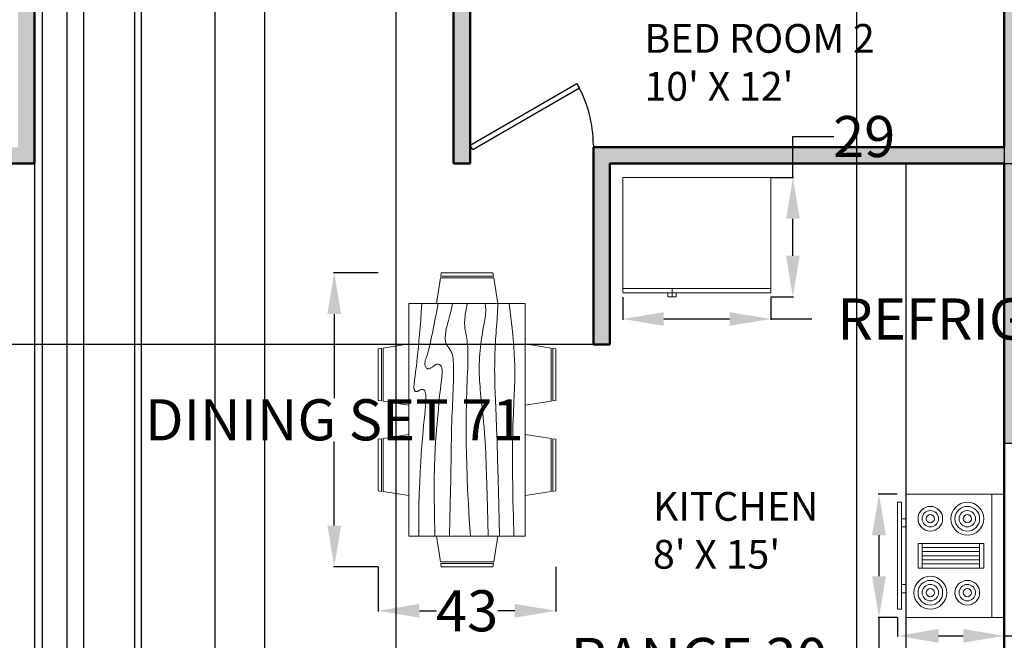
# Model space of a CAD drawing. Units: inches. Extents: x 133 to 758, y -29 to 543.
# Tile 5 of 7: x 386 to 626, y 235 to 386. Entities that reach past the tile are written whole.
import ezdxf

# ---------------------------------------------------------------- set-up
doc = ezdxf.new("R2010")
doc.units = ezdxf.units.IN
doc.header["$MEASUREMENT"] = 0
for name, color, linetype, lineweight in [('A-ANNO-DIMS', 2, 'Continuous', 18), ('A-AREA-IDEN', 7, 'Continuous', 25), ('A-EQPM', 8, 'Continuous', 20), ('A-FLOR-CASE', 32, 'Continuous', 25), ('A-FURN', 8, 'Continuous', 18), ('A-WALL', 7, 'Continuous', 50), ('DOOR', 40, 'Continuous', 25)]:
    doc.layers.add(name, color=color, linetype=linetype, lineweight=lineweight)
doc.layers.add('A-WALL-PATT', color=251, linetype='Continuous', lineweight=13, true_color=0x636466)
doc.styles.get("Standard").update_dxf_attribs({"font": 'arial.ttf'})
doc.dimstyles.get("Standard").update_dxf_attribs({"dimtxt": 10, "dimasz": 10, "dimexe": 0.18, "dimexo": 0.0625, "dimgap": 0.09, "dimtad": 0, "dimtih": 1, "dimtoh": 1, "dimdec": 0, "dimzin": 0, "dimdsep": 46, "dimlunit": 4, "dimtxsty": 'Standard', "dimcen": 0.09, "dimadec": 0, "dimazin": 0, "dimtfac": 1, "dimtdec": 0, "dimtofl": 0, "dimtmove": 0, "dimatfit": 3, "dimfxl": 1, "dimtolj": 1, "dimtzin": 0, "dimarcsym": 0})

# ---------------------------------------------------------------- blocks, each defined once
blk = doc.blocks.new('*U11')
for p, q in [((0, 0), (0, -6)), ((40, 0), (40, -6))]:
    blk.add_line(p, q)
blk.add_lwpolyline([(0, 0), (34.64, 20), (35.52, 18.48), (0.87, -1.52)], close=True)
blk.add_arc((0, 0), 40, 0, 30)
blk = doc.blocks.new('Range-Oven - 30 in top')
for p, q in [((0, -3), (30, -3)), ((12, -6), (18, -6)), ((13, -20), (13, -6)), ((14, -6), (14, -20)), ((15, -20), (15, -6)), ((16, -6), (16, -20)), ((17, -20), (17, -6)), ((18, -20), (12, -20)), ((6, -24), (6, -25)), ((8, -25), (8, -24)), ((22, -25), (22, -24)), ((24, -24), (24, -25))]:
    blk.add_line(p, q)
for points in [[(0, -24), (0, 0), (30, 0), (30, -24)], [(12, -21), (12, -5), (18, -5), (18, -21)], [(2, -26), (2, -25), (28, -25), (28, -26)]]:
    blk.add_lwpolyline(points, close=True)
for centre, radius in [((6, -9), 4), ((6, -9), 3), ((6, -9), 2), ((24, -9), 3), ((24, -9), 2), ((6, -9), 1), ((24, -9), 1), ((24, -18), 4), ((6, -18), 3), ((6, -18), 2), ((24, -18), 3), ((24, -18), 2), ((6, -18), 1), ((24, -18), 1)]:
    blk.add_circle(centre, radius)
blk = doc.blocks.new('Refrigerator-2 door - 36 in top')
for p, q in [((0, -26.999999), (36, -26.999999)), ((11, -27.999999), (11, -28.999999)), ((12, -26.999999), (12, -28.999999)), ((13, -28.999999), (13, -27.999999)), ((11, -28.999999), (13, -28.999999))]:
    blk.add_line(p, q)
blk.add_lwpolyline([(0, -27.999999), (0, 0), (36, 0), (36, -27.999999)], close=True)
blk = doc.blocks.new('Dining Set - 36 x 72 in.')
for p, q in [((-22, 27.5), (-22.1562, 26.50042)), ((-22, 27.5), (-6, 27.5)), ((-5.8437, 26.49966), (-6, 27.5)), ((6, 27.5), (5.8438, 26.50042)), ((6, 27.5), (22, 27.5)), ((22.1563, 26.49966), (22, 27.5)), ((-22.2343, 26.00059), (-23.4847, 17.99762)), ((-22.2304, 26), (-5.7608, 26)), ((-5.8416, 26.5), (-22.1534, 26.5)), ((-4.5152, 17.99762), (-5.7655, 25.99926)), ((5.7657, 26.00059), (4.5153, 17.99762)), ((5.7696, 26), (22.2392, 26)), ((22.1584, 26.5), (5.8466, 26.5)), ((23.4848, 17.99762), (22.2345, 25.99926)), ((36, 18), (-36, 18)), ((-36, 18), (-36, -18)), ((36, -18), (36, 18)), ((-44.0006, 8.23428), (-35.9976, 9.48474)), ((44.0006, 8.23428), (35.9976, 9.48474)), ((-45.5, 8), (-44.5004, 8.15617)), ((-45.5, 8), (-45.5, -8)), ((-44.5, -8.15843), (-44.5, 8.15338)), ((-44, 8.23041), (-44, -8.23915)), ((44, 8.23041), (44, -8.23915)), ((44.5, -8.15843), (44.5, 8.15338)), ((45.5, 8), (44.5005, 8.15617)), ((45.5, 8), (45.5, -8)), ((-44.4997, -8.15631), (-45.5, -8)), ((-35.9976, -9.48476), (-43.9993, -8.2345)), ((35.9976, -9.48476), (43.9993, -8.2345)), ((44.4997, -8.15631), (45.5, -8)), ((-36, -18), (36, -18)), ((-22.2343, -26.0006), (-23.4847, -17.99762)), ((-4.5152, -17.99762), (-5.7655, -25.99928)), ((5.7657, -26.0006), (4.5153, -17.99762)), ((23.4848, -17.99762), (22.2345, -25.99928)), ((-22.2304, -26), (-5.7608, -26)), ((-22, -27.5), (-22.1562, -26.50044)), ((-5.8416, -26.5), (-22.1534, -26.5)), ((-5.8437, -26.49967), (-6, -27.5)), ((5.7696, -26), (22.2392, -26)), ((6, -27.5), (5.8438, -26.50044)), ((22.1584, -26.5), (5.8466, -26.5)), ((22.1563, -26.49967), (22, -27.5)), ((-22, -27.5), (-6, -27.5)), ((6, -27.5), (22, -27.5))]:
    blk.add_line(p, q)
for points in [[(-36, 15), (-31.1772, 14.97754), (-26.8079, 14.91406), (-22.8538, 14.81543), (-19.276, 14.6875), (-16.0362, 14.53613), (-13.0957, 14.36718), (-10.4159, 14.18652), (-7.9583, 14), (-5.6904, 13.81315), (-3.6035, 13.63021), (-1.6954, 13.45508), (0.0365, 13.29166), (1.5945, 13.14388), (2.9811, 13.01562), (4.1988, 12.9108), (5.25, 12.83333), (6.1393, 12.78613), (6.8802, 12.76823), (7.4883, 12.77767), (7.9792, 12.8125), (8.3685, 12.87077), (8.6719, 12.95052), (8.9049, 13.0498), (9.0833, 13.16666), (9.2205, 13.29899), (9.3216, 13.44401), (9.3895, 13.59879), (9.4271, 13.76041), (9.4373, 13.92594), (9.4232, 14.09245), (9.3875, 14.257), (9.3333, 14.41666), (9.2638, 14.56917), (9.1836, 14.71484), (9.0975, 14.85465), (9.0104, 14.98958), (8.9272, 15.1206), (8.8529, 15.2487), (8.7922, 15.37483), (8.75, 15.5), (8.7305, 15.62467), (8.7344, 15.74739), (8.7617, 15.86621), (8.8125, 15.97916), (8.8867, 16.08431), (8.9844, 16.17968), (9.1055, 16.26334), (9.25, 16.33333), (9.4189, 16.38802), (9.6172, 16.42708), (9.8506, 16.45052), (10.125, 16.45833), (10.4463, 16.45052), (10.8203, 16.42708), (11.2529, 16.38802), (11.75, 16.33333), (12.3184, 16.26318), (12.9694, 16.17838), (13.7151, 16.07991), (14.5677, 15.96875), (15.5395, 15.84586), (16.6426, 15.71224), (17.8893, 15.56884), (19.2917, 15.41666), (20.859, 15.25667), (22.5879, 15.08984), (24.4721, 14.91715), (26.5052, 14.73958), (28.6809, 14.5581), (30.9929, 14.3737), (33.4347, 14.18733), (36, 14)], [(-36, 10), (-28.9766, 10.14274), (-23.1725, 10.20442), (-18.4241, 10.19775), (-14.5677, 10.13541), (-11.4399, 10.03011), (-8.877, 9.89453), (-6.7154, 9.74137), (-4.7917, 9.58333), (-2.9698, 9.43082), (-1.2246, 9.28515), (0.4415, 9.14534), (2.026, 9.01041), (3.5266, 8.87939), (4.9408, 8.7513), (6.266, 8.62516), (7.5, 8.5), (8.6411, 8.37549), (9.6914, 8.2539), (10.6538, 8.13818), (11.5312, 8.03125), (12.3267, 7.93603), (13.043, 7.85547), (13.6831, 7.79248), (14.25, 7.75), (14.7471, 7.7303), (15.1797, 7.73307), (15.5537, 7.75732), (15.875, 7.80208), (16.1494, 7.86637), (16.3828, 7.94922), (16.5811, 8.04964), (16.75, 8.16666), (16.8944, 8.29915), (17.0143, 8.44531), (17.1089, 8.60319), (17.1771, 8.77083), (17.218, 8.94629), (17.2305, 9.1276), (17.2137, 9.31282), (17.1667, 9.5), (17.0895, 9.6875), (16.987, 9.875), (16.8649, 10.0625), (16.7292, 10.25), (16.5856, 10.4375), (16.4401, 10.625), (16.2985, 10.8125), (16.1667, 11), (16.05, 11.18733), (15.9518, 11.3737), (15.8752, 11.5581), (15.8229, 11.73958), (15.798, 11.91715), (15.8034, 12.08984), (15.842, 12.25667), (15.9167, 12.41666), (16.0295, 12.56836), (16.1784, 12.70833), (16.3605, 12.83268), (16.5729, 12.9375), (16.8127, 13.01888), (17.0768, 13.07291), (17.3625, 13.0957), (17.6667, 13.08333), (17.9894, 13.03312), (18.3418, 12.94726), (18.7382, 12.82918), (19.1927, 12.68229), (19.7195, 12.51001), (20.3327, 12.31575), (21.0465, 12.10294), (21.875, 11.875), (22.8357, 11.63354), (23.959, 11.37304), (25.2786, 11.08618), (26.8282, 10.76562), (28.6414, 10.40405), (30.752, 9.99414), (33.1936, 9.52856), (36, 9)], [(-36, 5.5), (-30.7157, 5.3348), (-26.069, 5.20963), (-21.9946, 5.11767), (-18.4271, 5.05208), (-15.3009, 5.00602), (-12.5508, 4.97265), (-10.1112, 4.94515), (-7.9167, 4.91666), (-5.909, 4.88167), (-4.0586, 4.83984), (-2.3429, 4.79215), (-0.7396, 4.73958), (0.7739, 4.6831), (2.22, 4.6237), (3.6213, 4.56233), (5, 4.5), (6.373, 4.43782), (7.7344, 4.3776), (9.0723, 4.32129), (10.375, 4.27083), (11.6309, 4.22819), (12.8281, 4.19531), (13.9551, 4.17415), (15, 4.16666), (15.954, 4.17448), (16.819, 4.19791), (17.6001, 4.23698), (18.3021, 4.29166), (18.9299, 4.36198), (19.4883, 4.44791), (19.9823, 4.54948), (20.4167, 4.66666), (20.7969, 4.79899), (21.1302, 4.94401), (21.4245, 5.09879), (21.6875, 5.26041), (21.9271, 5.42594), (22.1511, 5.59245), (22.3672, 5.757), (22.5834, 5.91666), (22.8065, 6.06868), (23.0404, 6.21093), (23.2879, 6.34147), (23.5521, 6.45833), (23.8358, 6.55957), (24.142, 6.64323), (24.4735, 6.70735), (24.8334, 6.75), (25.2235, 6.76969), (25.642, 6.76692), (26.0858, 6.74267), (26.5521, 6.69791), (27.0379, 6.63362), (27.5404, 6.55078), (28.0565, 6.45036), (28.5834, 6.33333), (29.1242, 6.19987), (29.7071, 6.04687), (30.3661, 5.87044), (31.1354, 5.66666), (32.0493, 5.43164), (33.142, 5.16146), (34.4475, 4.85221), (36, 4.5)], [(-36, -1), (-30.7915, -0.6591), (-26.0195, -0.38216), (-21.6519, -0.16284), (-17.6563, 0.00521), (-14.0005, 0.12833), (-10.6523, 0.21289), (-7.5796, 0.26522), (-4.75, 0.29166), (-2.134, 0.29793), (0.2878, 0.28711), (2.5317, 0.26163), (4.6146, 0.22396), (6.5529, 0.17651), (8.3633, 0.12174), (10.0623, 0.06209), (11.6667, 0), (13.1899, -0.06201), (14.6341, -0.1211), (15.9982, -0.17432), (17.2813, -0.21875), (18.4823, -0.25147), (19.6003, -0.26953), (20.6343, -0.27002), (21.5834, -0.25), (22.4481, -0.20768), (23.2357, -0.14584), (23.9549, -0.06836), (24.6146, 0.02083), (25.2235, 0.11784), (25.7904, 0.21875), (26.3241, 0.31966), (26.8334, 0.41666), (27.3265, 0.50618), (27.8099, 0.58593), (28.2894, 0.65397), (28.7709, 0.70833), (29.2601, 0.74707), (29.763, 0.76823), (30.2855, 0.76985), (30.8334, 0.75), (31.4088, 0.70784), (31.9994, 0.64713), (32.589, 0.57275), (33.1615, 0.48958), (33.7008, 0.4025), (34.1908, 0.3164), (34.6153, 0.23616), (34.9584, 0.16666), (35.2099, 0.11165), (35.3848, 0.07031), (35.504, 0.04069), (35.5886, 0.02083), (35.6594, 0.00879), (35.7377, 0.0026), (35.8442, 0.00032), (36, 0)], [(-36, -6.5), (-27.1843, -6.31267), (-20.084, -6.1263), (-14.469, -5.9419), (-10.1094, -5.76042), (-6.7752, -5.58285), (-4.2363, -5.41016), (-2.2629, -5.24333), (-0.625, -5.08334), (0.8708, -4.93099), (2.2715, -4.78646), (3.5872, -4.64974), (4.8281, -4.52084), (6.0046, -4.39974), (7.127, -4.28646), (8.2053, -4.18099), (9.25, -4.08334), (10.2705, -3.99382), (11.2734, -3.91407), (12.2647, -3.84603), (13.25, -3.79167), (14.2354, -3.75293), (15.2266, -3.73177), (16.2295, -3.73015), (17.25, -3.75), (18.2912, -3.79248), (19.3451, -3.85547), (20.4009, -3.93604), (21.4479, -4.03125), (22.4754, -4.13819), (23.4727, -4.25391), (24.4289, -4.37549), (25.3334, -4.5), (26.1785, -4.62492), (26.9694, -4.74935), (27.7145, -4.87281), (28.4219, -4.99479), (29.1, -5.11483), (29.7572, -5.23242), (30.4016, -5.34709), (31.0417, -5.45834), (31.6837, -5.56437), (32.3262, -5.65821), (32.9658, -5.73153), (33.599, -5.77604), (34.2224, -5.78345), (34.8327, -5.74545), (35.4264, -5.65373), (36, -5.5)], [(-36, -10), (-26.4022, -9.81299), (-18.4675, -9.62891), (-11.9839, -9.45069), (-6.7396, -9.28125), (-2.5226, -9.12354), (0.8789, -8.98047), (3.6769, -8.85498), (6.0833, -8.75), (8.2767, -8.66765), (10.3021, -8.60677), (12.1712, -8.56543), (13.8958, -8.54167), (15.4876, -8.53353), (16.9583, -8.53907), (18.3197, -8.55632), (19.5834, -8.58334), (20.7616, -8.61841), (21.8685, -8.66081), (22.9188, -8.71004), (23.9271, -8.76563), (24.9081, -8.82707), (25.8763, -8.89388), (26.8465, -8.96558), (27.8334, -9.04167), (28.8474, -9.12118), (29.8828, -9.20117), (30.93, -9.27824), (31.9792, -9.34896), (33.0205, -9.40991), (34.0443, -9.45768), (35.0407, -9.48885), (36, -9.5)], [(-36, -14.5), (-30.0881, -14.33513), (-25.0332, -14.21224), (-20.7312, -14.12647), (-17.0781, -14.07292), (-13.97, -14.04671), (-11.3027, -14.04297), (-8.9724, -14.05681), (-6.875, -14.08334), (-4.9224, -14.11833), (-3.0905, -14.16016), (-1.3709, -14.20785), (0.2448, -14.26042), (1.7647, -14.3169), (3.1973, -14.3763), (4.5507, -14.43767), (5.8333, -14.5), (7.0554, -14.5621), (8.235, -14.62175), (9.3922, -14.67652), (10.5469, -14.72396), (11.7192, -14.76164), (12.929, -14.78711), (14.1965, -14.79794), (15.5417, -14.79167), (16.9933, -14.76424), (18.6152, -14.70508), (20.4804, -14.60197), (22.6615, -14.44271), (25.2312, -14.21509), (28.2624, -13.9069), (31.8277, -13.50594), (36, -13)]]:
    blk.add_lwpolyline(points)
blk = doc.blocks.new('*D44')
at = {"layer": 'A-ANNO-DIMS', "color": 0, "lineweight": -2, "transparency": 16777216}
for p, q in [((538.86, 405.84), (538.86, 393.72)), ((618.86, 405.84), (618.86, 393.72)), ((548.86, 393.9), (608.86, 393.9)), ((618.86, 393.9), (628.86, 393.9))]:
    blk.add_line(p, q, dxfattribs=at)
at = {"layer": 'A-ANNO-DIMS', "color": 0, "transparency": 16777216}
for points in [[(548.86, 395.56), (548.86, 392.23), (538.86, 393.9)], [(608.86, 395.56), (608.86, 392.23), (618.86, 393.9)]]:
    blk.add_solid(points, dxfattribs=at)
at = {"layer": 'Defpoints', "color": 0, "transparency": 16777216}
for p in [(538.86, 405.9), (618.86, 405.9), (618.86, 393.9)]:
    blk.add_point(p, dxfattribs=at)
at = {"layer": 'A-ANNO-DIMS', "color": 0, "transparency": 16777216, "insert": (696.36, 393.9), "char_height": 10, "attachment_point": 5}
blk.add_mtext('\\A1;QUEEN BED 80 TYP.', dxfattribs=at)
blk = doc.blocks.new('*D62')
at = {"layer": 'A-ANNO-DIMS', "color": 0, "lineweight": -2, "transparency": 16777216}
for p, q in [((599.69, 270.92), (595.07, 270.92)), ((595.25, 260.92), (595.25, 250.92)), ((599.69, 240.92), (595.07, 240.92)), ((595.25, 240.92), (595.25, 230.92)), ((595.25, 230.92), (585.25, 230.92))]:
    blk.add_line(p, q, dxfattribs=at)
at = {"layer": 'A-ANNO-DIMS', "color": 0, "transparency": 16777216}
for points in [[(593.58, 260.92), (596.92, 260.92), (595.25, 270.92)], [(593.58, 250.92), (596.92, 250.92), (595.25, 240.92)]]:
    blk.add_solid(points, dxfattribs=at)
at = {"layer": 'Defpoints', "color": 0, "transparency": 16777216}
for p in [(599.75, 270.92), (595.25, 240.92), (599.75, 240.92)]:
    blk.add_point(p, dxfattribs=at)
at = {"layer": 'A-ANNO-DIMS', "color": 0, "transparency": 16777216, "insert": (551.49, 230.92), "char_height": 10, "attachment_point": 5}
blk.add_mtext('\\A1;RANGE 30', dxfattribs=at)
blk = doc.blocks.new('*D63')
at = {"layer": 'A-ANNO-DIMS', "color": 0, "lineweight": -2, "transparency": 16777216}
for p, q in [((599.75, 240.86), (599.75, 236.24)), ((625.75, 240.86), (625.75, 236.24)), ((609.75, 236.42), (615.75, 236.42)), ((625.75, 236.42), (635.75, 236.42))]:
    blk.add_line(p, q, dxfattribs=at)
at = {"layer": 'A-ANNO-DIMS', "color": 0, "transparency": 16777216}
for points in [[(609.75, 238.09), (609.75, 234.75), (599.75, 236.42)], [(615.75, 238.09), (615.75, 234.75), (625.75, 236.42)]]:
    blk.add_solid(points, dxfattribs=at)
at = {"layer": 'Defpoints', "color": 0, "transparency": 16777216}
for p in [(599.75, 240.92), (625.75, 240.92), (625.75, 236.42)]:
    blk.add_point(p, dxfattribs=at)
at = {"layer": 'A-ANNO-DIMS', "color": 0, "transparency": 16777216, "insert": (643.08, 236.42), "char_height": 10, "attachment_point": 5}
blk.add_mtext('\\A1;26', dxfattribs=at)
blk = doc.blocks.new('*D66')
at = {"layer": 'A-ANNO-DIMS', "color": 0, "lineweight": -2, "transparency": 16777216}
for p, q in [((532.9, 318.87), (532.9, 313.35)), ((568.9, 318.87), (568.9, 313.35)), ((542.9, 313.53), (558.9, 313.53)), ((568.9, 313.53), (578.9, 313.53))]:
    blk.add_line(p, q, dxfattribs=at)
at = {"layer": 'A-ANNO-DIMS', "color": 0, "transparency": 16777216}
for points in [[(542.9, 315.2), (542.9, 311.86), (532.9, 313.53)], [(558.9, 315.2), (558.9, 311.86), (568.9, 313.53)]]:
    blk.add_solid(points, dxfattribs=at)
at = {"layer": 'Defpoints', "color": 0, "transparency": 16777216}
for p in [(532.9, 318.93), (568.9, 318.93), (568.9, 313.53)]:
    blk.add_point(p, dxfattribs=at)
at = {"layer": 'A-ANNO-DIMS', "color": 0, "transparency": 16777216, "insert": (643.33, 313.53), "char_height": 10, "attachment_point": 5}
blk.add_mtext('\\A1;REFRIGERATOR 36', dxfattribs=at)
blk = doc.blocks.new('*D67')
at = {"layer": 'A-ANNO-DIMS', "color": 0, "lineweight": -2, "transparency": 16777216}
for p, q in [((574.3, 347.93), (574.3, 357.93)), ((574.3, 357.93), (584.3, 357.93)), ((568.97, 347.93), (574.48, 347.93)), ((574.3, 328.93), (574.3, 337.93)), ((568.97, 318.93), (574.48, 318.93))]:
    blk.add_line(p, q, dxfattribs=at)
at = {"layer": 'A-ANNO-DIMS', "color": 0, "transparency": 16777216}
for points in [[(572.64, 337.93), (575.97, 337.93), (574.3, 347.93)], [(572.64, 328.93), (575.97, 328.93), (574.3, 318.93)]]:
    blk.add_solid(points, dxfattribs=at)
at = {"layer": 'Defpoints', "color": 0, "transparency": 16777216}
for p in [(568.9, 347.93), (574.3, 347.93), (568.9, 318.93)]:
    blk.add_point(p, dxfattribs=at)
at = {"layer": 'A-ANNO-DIMS', "color": 0, "transparency": 16777216, "insert": (591.65, 357.93), "char_height": 10, "attachment_point": 5}
blk.add_mtext('\\A1;29', dxfattribs=at)
blk = doc.blocks.new('*D68')
at = {"layer": 'A-ANNO-DIMS', "color": 0, "lineweight": -2, "transparency": 16777216}
for p, q in [((473.36, 324.74), (462.52, 324.74)), ((462.7, 314.74), (462.7, 294.25)), ((462.7, 263.25), (462.7, 283.73)), ((473.36, 253.25), (462.52, 253.25))]:
    blk.add_line(p, q, dxfattribs=at)
at = {"layer": 'A-ANNO-DIMS', "color": 0, "transparency": 16777216}
for points in [[(461.04, 314.74), (464.37, 314.74), (462.7, 324.74)], [(461.04, 263.25), (464.37, 263.25), (462.7, 253.25)]]:
    blk.add_solid(points, dxfattribs=at)
at = {"layer": 'Defpoints', "color": 0, "transparency": 16777216}
for p in [(462.7, 324.74), (473.43, 324.74), (473.43, 253.25)]:
    blk.add_point(p, dxfattribs=at)
at = {"layer": 'A-ANNO-DIMS', "color": 0, "transparency": 16777216, "insert": (462.7, 288.99), "char_height": 10, "attachment_point": 5}
blk.add_mtext('\\A1;DINING SET 71', dxfattribs=at)
blk = doc.blocks.new('*D69')
at = {"layer": 'A-ANNO-DIMS', "color": 0, "lineweight": -2, "transparency": 16777216}
for p, q in [((473.43, 253.18), (473.43, 242.34)), ((516.64, 253.18), (516.64, 242.34)), ((483.43, 242.52), (487.58, 242.52)), ((506.64, 242.52), (502.49, 242.52))]:
    blk.add_line(p, q, dxfattribs=at)
at = {"layer": 'A-ANNO-DIMS', "color": 0, "transparency": 16777216}
for points in [[(483.43, 244.19), (483.43, 240.85), (473.43, 242.52)], [(506.64, 244.19), (506.64, 240.85), (516.64, 242.52)]]:
    blk.add_solid(points, dxfattribs=at)
at = {"layer": 'Defpoints', "color": 0, "transparency": 16777216}
for p in [(473.43, 253.25), (516.64, 253.25), (473.43, 242.52)]:
    blk.add_point(p, dxfattribs=at)
at = {"layer": 'A-ANNO-DIMS', "color": 0, "transparency": 16777216, "insert": (495.03, 242.52), "char_height": 10, "attachment_point": 5}
blk.add_mtext('\\A1;43', dxfattribs=at)
blk = doc.blocks.new('*D75')
at = {"layer": 'A-ANNO-DIMS', "color": 0, "lineweight": -2, "transparency": 16777216}
for p, q in [((525.69, 307.34), (231.17, 307.34)), ((231.35, 297.34), (231.35, 264.53)), ((231.35, 221.34), (231.35, 254.14)), ((525.69, 211.34), (231.17, 211.34))]:
    blk.add_line(p, q, dxfattribs=at)
at = {"layer": 'A-ANNO-DIMS', "color": 0, "transparency": 16777216}
for points in [[(229.68, 297.34), (233.02, 297.34), (231.35, 307.34)], [(229.68, 221.34), (233.02, 221.34), (231.35, 211.34)]]:
    blk.add_solid(points, dxfattribs=at)
at = {"layer": 'Defpoints', "color": 0, "transparency": 16777216}
for p in [(231.35, 307.34), (525.75, 307.34), (525.75, 211.34)]:
    blk.add_point(p, dxfattribs=at)
at = {"layer": 'A-ANNO-DIMS', "color": 0, "transparency": 16777216, "insert": (231.35, 259.34), "char_height": 10, "attachment_point": 5}
blk.add_mtext('\\A1;96', dxfattribs=at)
blk = doc.blocks.new('*D78')
at = {"layer": 'A-ANNO-DIMS', "color": 0, "lineweight": -2, "transparency": 16777216}
for p, q in [((361.75, 167.4), (361.75, 533.92)), ((371.75, 533.74), (381.75, 533.74)), ((391.75, 167.4), (391.75, 533.92)), ((391.75, 533.74), (401.75, 533.74))]:
    blk.add_line(p, q, dxfattribs=at)
at = {"layer": 'A-ANNO-DIMS', "color": 0, "transparency": 16777216}
for points in [[(371.75, 535.4), (371.75, 532.07), (361.75, 533.74)], [(381.75, 535.4), (381.75, 532.07), (391.75, 533.74)]]:
    blk.add_solid(points, dxfattribs=at)
at = {"layer": 'Defpoints', "color": 0, "transparency": 16777216}
for p in [(391.75, 533.74), (361.75, 167.34), (391.75, 167.34)]:
    blk.add_point(p, dxfattribs=at)
at = {"layer": 'A-ANNO-DIMS', "color": 0, "transparency": 16777216, "insert": (408.98, 533.74), "char_height": 10, "attachment_point": 5}
blk.add_mtext('\\A1;30', dxfattribs=at)
blk = doc.blocks.new('*D81')
at = {"layer": 'A-ANNO-DIMS', "color": 0, "lineweight": -2, "transparency": 16777216}
for p, q in [((589.75, 499.27), (589.75, -22.24)), ((625.75, 499.27), (625.75, -22.24)), ((599.75, -22.06), (600.5, -22.06)), ((615.75, -22.06), (615, -22.06))]:
    blk.add_line(p, q, dxfattribs=at)
at = {"layer": 'A-ANNO-DIMS', "color": 0, "transparency": 16777216}
for points in [[(599.75, -20.4), (599.75, -23.73), (589.75, -22.06)], [(615.75, -20.4), (615.75, -23.73), (625.75, -22.06)]]:
    blk.add_solid(points, dxfattribs=at)
at = {"layer": 'Defpoints', "color": 0, "transparency": 16777216}
for p in [(589.75, 499.34), (625.75, 499.34), (625.75, -22.06)]:
    blk.add_point(p, dxfattribs=at)
at = {"layer": 'A-ANNO-DIMS', "color": 0, "transparency": 16777216, "insert": (607.75, -22.06), "char_height": 10, "attachment_point": 5}
blk.add_mtext('\\A1;36', dxfattribs=at)
blk = doc.blocks.new('*D82')
at = {"layer": 'A-ANNO-DIMS', "color": 0, "lineweight": -2, "transparency": 16777216}
for p, q in [((625.81, 351.34), (660.33, 351.34)), ((660.15, 341.34), (660.15, 322.53)), ((660.15, 293.34), (660.15, 312.14)), ((625.81, 283.34), (660.33, 283.34))]:
    blk.add_line(p, q, dxfattribs=at)
at = {"layer": 'A-ANNO-DIMS', "color": 0, "transparency": 16777216}
for points in [[(658.48, 341.34), (661.82, 341.34), (660.15, 351.34)], [(658.48, 293.34), (661.82, 293.34), (660.15, 283.34)]]:
    blk.add_solid(points, dxfattribs=at)
at = {"layer": 'Defpoints', "color": 0, "transparency": 16777216}
for p in [(625.75, 351.34), (625.75, 283.34), (660.15, 283.34)]:
    blk.add_point(p, dxfattribs=at)
at = {"layer": 'A-ANNO-DIMS', "color": 0, "transparency": 16777216, "insert": (660.15, 317.34), "char_height": 10, "attachment_point": 5}
blk.add_mtext('\\A1;68', dxfattribs=at)
blk = doc.blocks.new('*D85')
at = {"layer": 'A-ANNO-DIMS', "color": 0, "lineweight": -2, "transparency": 16777216}
for p, q in [((389.75, 399.27), (389.75, -22.24)), ((415.75, 399.27), (415.75, -22.24)), ((389.75, -22.06), (379.75, -22.06)), ((405.75, -22.06), (399.75, -22.06))]:
    blk.add_line(p, q, dxfattribs=at)
at = {"layer": 'A-ANNO-DIMS', "color": 0, "transparency": 16777216}
for points in [[(399.75, -20.4), (399.75, -23.73), (389.75, -22.06)], [(405.75, -20.4), (405.75, -23.73), (415.75, -22.06)]]:
    blk.add_solid(points, dxfattribs=at)
at = {"layer": 'Defpoints', "color": 0, "transparency": 16777216}
for p in [(389.75, 399.34), (415.75, 399.34), (389.75, -22.06)]:
    blk.add_point(p, dxfattribs=at)
at = {"layer": 'A-ANNO-DIMS', "color": 0, "transparency": 16777216, "insert": (372.42, -22.06), "char_height": 10, "attachment_point": 5}
blk.add_mtext('\\A1;26', dxfattribs=at)
blk = doc.blocks.new('*D89')
at = {"layer": 'A-ANNO-DIMS', "color": 0, "lineweight": -2, "transparency": 16777216}
for p, q in [((387.75, 533.74), (377.75, 533.74)), ((397.75, 163.4), (397.75, 533.92)), ((401.75, 163.4), (401.75, 533.92)), ((411.75, 533.74), (421.75, 533.74))]:
    blk.add_line(p, q, dxfattribs=at)
at = {"layer": 'A-ANNO-DIMS', "color": 0, "transparency": 16777216}
for points in [[(387.75, 535.4), (387.75, 532.07), (397.75, 533.74)], [(411.75, 535.4), (411.75, 532.07), (401.75, 533.74)]]:
    blk.add_solid(points, dxfattribs=at)
at = {"layer": 'Defpoints', "color": 0, "transparency": 16777216}
for p in [(401.75, 533.74), (397.75, 163.34), (401.75, 163.34)]:
    blk.add_point(p, dxfattribs=at)
at = {"layer": 'A-ANNO-DIMS', "color": 0, "transparency": 16777216, "insert": (425.3, 533.74), "char_height": 10, "attachment_point": 5}
blk.add_mtext('\\A1;4', dxfattribs=at)
blk = doc.blocks.new('*D90')
at = {"layer": 'A-ANNO-DIMS', "color": 0, "lineweight": -2, "transparency": 16777216}
for p, q in [((433.75, 167.4), (433.75, 533.92)), ((443.75, 533.74), (448.32, 533.74)), ((467.75, 533.74), (463.18, 533.74)), ((477.75, 163.4), (477.75, 533.92))]:
    blk.add_line(p, q, dxfattribs=at)
at = {"layer": 'A-ANNO-DIMS', "color": 0, "transparency": 16777216}
for points in [[(443.75, 535.4), (443.75, 532.07), (433.75, 533.74)], [(467.75, 535.4), (467.75, 532.07), (477.75, 533.74)]]:
    blk.add_solid(points, dxfattribs=at)
at = {"layer": 'Defpoints', "color": 0, "transparency": 16777216}
for p in [(477.75, 533.74), (433.75, 167.34), (477.75, 163.34)]:
    blk.add_point(p, dxfattribs=at)
at = {"layer": 'A-ANNO-DIMS', "color": 0, "transparency": 16777216, "insert": (455.75, 533.74), "char_height": 10, "attachment_point": 5}
blk.add_mtext('\\A1;44', dxfattribs=at)
blk = doc.blocks.new('*D91')
at = {"layer": 'A-ANNO-DIMS', "color": 0, "lineweight": -2, "transparency": 16777216}
for p, q in [((415.75, 399.27), (415.75, -22.24)), ((445.75, 399.27), (445.75, -22.24)), ((425.75, -22.06), (435.75, -22.06)), ((445.75, -22.06), (455.75, -22.06))]:
    blk.add_line(p, q, dxfattribs=at)
at = {"layer": 'A-ANNO-DIMS', "color": 0, "transparency": 16777216}
for points in [[(425.75, -20.4), (425.75, -23.73), (415.75, -22.06)], [(435.75, -20.4), (435.75, -23.73), (445.75, -22.06)]]:
    blk.add_solid(points, dxfattribs=at)
at = {"layer": 'Defpoints', "color": 0, "transparency": 16777216}
for p in [(415.75, 399.34), (445.75, 399.34), (445.75, -22.06)]:
    blk.add_point(p, dxfattribs=at)
at = {"layer": 'A-ANNO-DIMS', "color": 0, "transparency": 16777216, "insert": (462.98, -22.06), "char_height": 10, "attachment_point": 5}
blk.add_mtext('\\A1;30', dxfattribs=at)
blk = doc.blocks.new('*D99')
at = {"layer": 'A-ANNO-DIMS', "color": 0, "lineweight": -2, "transparency": 16777216}
for p, q in [((391.75, 533.74), (381.75, 533.74)), ((401.75, 19.4), (401.75, 533.92)), ((414.17, 21.95), (414.17, 533.92)), ((424.17, 533.74), (434.17, 533.74))]:
    blk.add_line(p, q, dxfattribs=at)
at = {"layer": 'A-ANNO-DIMS', "color": 0, "transparency": 16777216}
for points in [[(391.75, 535.4), (391.75, 532.07), (401.75, 533.74)], [(424.17, 535.4), (424.17, 532.07), (414.17, 533.74)]]:
    blk.add_solid(points, dxfattribs=at)
at = {"layer": 'Defpoints', "color": 0, "transparency": 16777216}
for p in [(401.75, 533.74), (414.17, 21.89), (401.75, 19.34)]:
    blk.add_point(p, dxfattribs=at)
at = {"layer": 'A-ANNO-DIMS', "color": 0, "transparency": 16777216, "insert": (361.37, 533.74), "char_height": 10, "attachment_point": 5}
blk.add_mtext('\\A1;12.417', dxfattribs=at)

msp = doc.modelspace()

# ---------------------------------------------------------------- hatches: boundary and pattern name
at = {"layer": 'A-WALL-PATT'}
h = msp.add_hatch(color=256, dxfattribs=at)
h.dxf.hatch_style = 1
h.paths.add_polyline_path([(433.7501, 508.336), (349.7501, 508.336), (349.7501, 499.336), (385.7501, 499.336), (385.7501, 403.336), (385.7501, 355.336), (379.7501, 355.336), (379.7501, 351.336), (389.7501, 351.336), (389.7501, 399.336), (415.7501, 399.336), (415.7501, 403.336), (389.7501, 403.336), (389.7501, 499.336), (433.7501, 499.336)])
h.paths.add_polyline_path([(541.7501, 508.336), (457.7501, 508.336), (457.7501, 499.336), (491.7501, 499.336), (491.7501, 403.336), (445.7501, 403.336), (445.7501, 399.336), (491.7501, 399.336), (491.7501, 351.336), (495.7501, 351.336), (495.7501, 399.336), (495.7501, 499.336), (513.7501, 499.336), (541.7501, 499.336)])
h.paths.add_polyline_path([(634.7501, 508.336), (589.7501, 508.336), (589.7501, 499.336), (625.7501, 499.336), (625.7501, 355.336), (525.7501, 355.336), (525.7501, 351.336), (525.7501, 307.336), (529.7501, 307.336), (529.7501, 351.336), (625.7501, 351.336), (625.7501, 283.336), (634.7501, 283.336)])
h.paths.add_polyline_path([(301.7501, 508.336), (256.7501, 508.336), (256.7501, 283.336), (265.7501, 283.336), (265.7501, 351.336), (349.7501, 351.336), (349.7501, 355.336), (265.7501, 355.336), (265.7501, 499.336), (301.7501, 499.336)])
h.paths.add_polyline_path([(361.7501, 167.336), (265.7501, 167.336), (265.7501, 235.336), (256.7501, 235.336), (256.7501, 10.336), (309.4362, 10.336), (309.4362, 19.336), (265.7501, 19.336), (265.7501, 163.336), (283.7501, 163.336), (361.7501, 163.336)])

# ---------------------------------------------------------------- linework, layer by layer
at = {"layer": 'A-FLOR-CASE'}
msp.add_line((601.7501, 351.336), (601.7501, 191.336), dxfattribs=at)
at = {"layer": 'A-WALL'}
for p, q in [((625.7501, 499.336), (625.7501, 355.336)), ((389.7501, 351.336), (389.7501, 399.336)), ((491.7501, 399.336), (491.7501, 351.336)), ((495.7501, 399.336), (495.7501, 351.336)), ((525.7501, 355.336), (625.7501, 355.336)), ((525.7501, 351.336), (525.7501, 355.336)), ((379.7501, 351.336), (389.7501, 351.336)), ((495.7501, 351.336), (491.7501, 351.336)), ((525.7501, 351.336), (525.7501, 307.336)), ((529.7501, 351.336), (529.7501, 307.336)), ((529.7501, 351.336), (625.7501, 351.336)), ((625.7501, 351.336), (625.7501, 167.336)), ((529.7501, 307.336), (525.7501, 307.336))]:
    msp.add_line(p, q, dxfattribs=at)

# ---------------------------------------------------------------- block references
at = {"layer": 'A-EQPM'}
msp.add_blockref('Refrigerator-2 door - 36 in top', (532.9033, 347.9301), dxfattribs=at)
at = {"layer": 'A-EQPM', "rotation": 270}
msp.add_blockref('Range-Oven - 30 in top', (625.7501, 270.9203), dxfattribs=at)
at = {"layer": 'A-FURN', "xscale": 0.7856607656645157, "yscale": 0.7856607656645157, "zscale": 0.7856607656645157, "rotation": 90}
msp.add_blockref('Dining Set - 36 x 72 in.', (495.0322, 288.9927), dxfattribs=at)
at = {"layer": 'DOOR', "xscale": 0.75, "yscale": 0.75, "zscale": 0.75}
msp.add_blockref('*U11', (495.7501, 355.836), dxfattribs=at)

# ---------------------------------------------------------------- texts
at = {"layer": 'A-AREA-IDEN', "char_height": 7, "attachment_point": 1}
for s, width, insert in [("BED ROOM 2 \\P10' X 12'", 109.09065, (538.1884, 385.3115)), ("KITCHEN\\P8' X 15'", 62.727145, (540.2554, 271.4286))]:
    msp.add_mtext_dynamic_manual_height_columns(s, width=width, gutter_width=1, heights=[0], dxfattribs=dict(at, insert=insert))

# ---------------------------------------------------------------- dimensions: what is measured, and where the dimension line sits
at = {"layer": 'A-ANNO-DIMS'}
for base, p1, p2, override, picture, middle in [((401.75012, 533.73604), (414.16755, 21.88596), (401.75012, 19.33604), {"dimdec": 3, "dimlfac": 1, "dimrnd": 0, "dimzin": 0, "dimdsep": 46, "dimlunit": 2}, '*D99', (361.37362, 533.73604)), ((391.7501, 533.736), (361.7501, 167.336), (391.7501, 167.336), {"dimdec": 0, "dimlfac": 1, "dimrnd": 0, "dimzin": 0, "dimdsep": 46, "dimlunit": 2}, '*D78', (408.982, 533.736)), ((401.7501, 533.736), (397.7501, 163.336), (401.7501, 163.336), {"dimdec": 0, "dimlfac": 1, "dimrnd": 0, "dimzin": 0, "dimdsep": 46, "dimlunit": 2}, '*D89', (425.2985, 533.736)), ((477.7501, 533.736), (433.7501, 167.336), (477.7501, 163.336), {"dimdec": 0, "dimlfac": 1, "dimrnd": 0, "dimzin": 0, "dimdsep": 46, "dimlunit": 2}, '*D90', (455.7501, 533.736)), ((625.7501, -22.064), (589.7501, 499.336), (625.7501, 499.336), {"dimdec": 0, "dimlfac": 1, "dimrnd": 0, "dimzin": 0, "dimdsep": 46, "dimlunit": 2}, '*D81', (607.7501, -22.064)), ((389.7501, -22.064), (415.7501, 399.336), (389.7501, 399.336), {"dimdec": 0, "dimlfac": 1, "dimrnd": 0, "dimzin": 0, "dimdsep": 46, "dimlunit": 2}, '*D85', (372.4159, -22.064)), ((445.7501, -22.064), (415.7501, 399.336), (445.7501, 399.336), {"dimdec": 0, "dimlfac": 1, "dimrnd": 0, "dimzin": 0, "dimdsep": 46, "dimlunit": 2}, '*D91', (462.982, -22.064)), ((625.7501, 236.4203), (599.7501, 240.9203), (625.7501, 240.9203), {"dimdec": 0, "dimlfac": 1, "dimrnd": 0, "dimzin": 0, "dimdsep": 46, "dimlunit": 2}, '*D63', (643.0843, 236.4203))]:
    dim = msp.add_linear_dim(base=base, p1=p1, p2=p2, dimstyle='Standard', override=override, dxfattribs=at)
    dim.commit()
    dim.dimension.update_dxf_attribs({"geometry": picture, "text_midpoint": middle})
for base, p1, p2, text, picture, middle in [((618.8575, 393.8976), (538.8574, 405.8976), (618.8575, 405.8976), 'QUEEN BED <> TYP.', '*D44', (696.3588, 393.8976)), ((568.9033, 313.5301), (532.9033, 318.9301), (568.9033, 318.9301), 'REFRIGERATOR <>', '*D66', (643.3282, 313.5301))]:
    dim = msp.add_linear_dim(base=base, p1=p1, p2=p2, text=text, dimstyle='Standard', override={"dimdec": 0, "dimlfac": 1, "dimrnd": 0, "dimzin": 0, "dimdsep": 46, "dimlunit": 2}, dxfattribs=at)
    dim.commit()
    dim.dimension.update_dxf_attribs({"geometry": picture, "text_midpoint": middle})
for base, p1, p2, angle, picture, middle in [((574.3033, 347.9301), (568.9033, 318.9301), (568.9033, 347.9301), 90, '*D67', (591.6511, 357.9301)), ((660.1501, 283.336), (625.7501, 351.336), (625.7501, 283.336), 90, '*D82', (660.1501, 317.336)), ((231.3501, 307.336), (525.7501, 211.336), (525.7501, 307.336), 90, '*D75', (231.3501, 259.336)), ((473.4265, 242.5208), (516.6379, 253.2451), (473.4265, 253.2451), 180, '*D69', (495.0322, 242.5208))]:
    dim = msp.add_linear_dim(base=base, p1=p1, p2=p2, angle=angle, dimstyle='Standard', override={"dimdec": 0, "dimlfac": 1, "dimrnd": 0, "dimzin": 0, "dimdsep": 46, "dimlunit": 2}, dxfattribs=at)
    dim.commit()
    dim.dimension.update_dxf_attribs({"geometry": picture, "text_midpoint": middle})
for base, p1, p2, angle, text, picture, middle in [((462.7023, 324.7402), (473.4265, 253.2451), (473.4265, 324.7402), 90, 'DINING SET <>', '*D68', (462.7023, 288.9927)), ((595.2501, 240.9203), (599.7501, 270.9203), (599.7501, 240.9203), 270, 'RANGE <>', '*D62', (551.4937, 230.9203))]:
    dim = msp.add_linear_dim(base=base, p1=p1, p2=p2, angle=angle, text=text, dimstyle='Standard', override={"dimdec": 0, "dimlfac": 1, "dimrnd": 0, "dimzin": 0, "dimdsep": 46, "dimlunit": 2}, dxfattribs=at)
    dim.commit()
    dim.dimension.update_dxf_attribs({"geometry": picture, "text_midpoint": middle})

doc.saveas('drawing.dxf')
